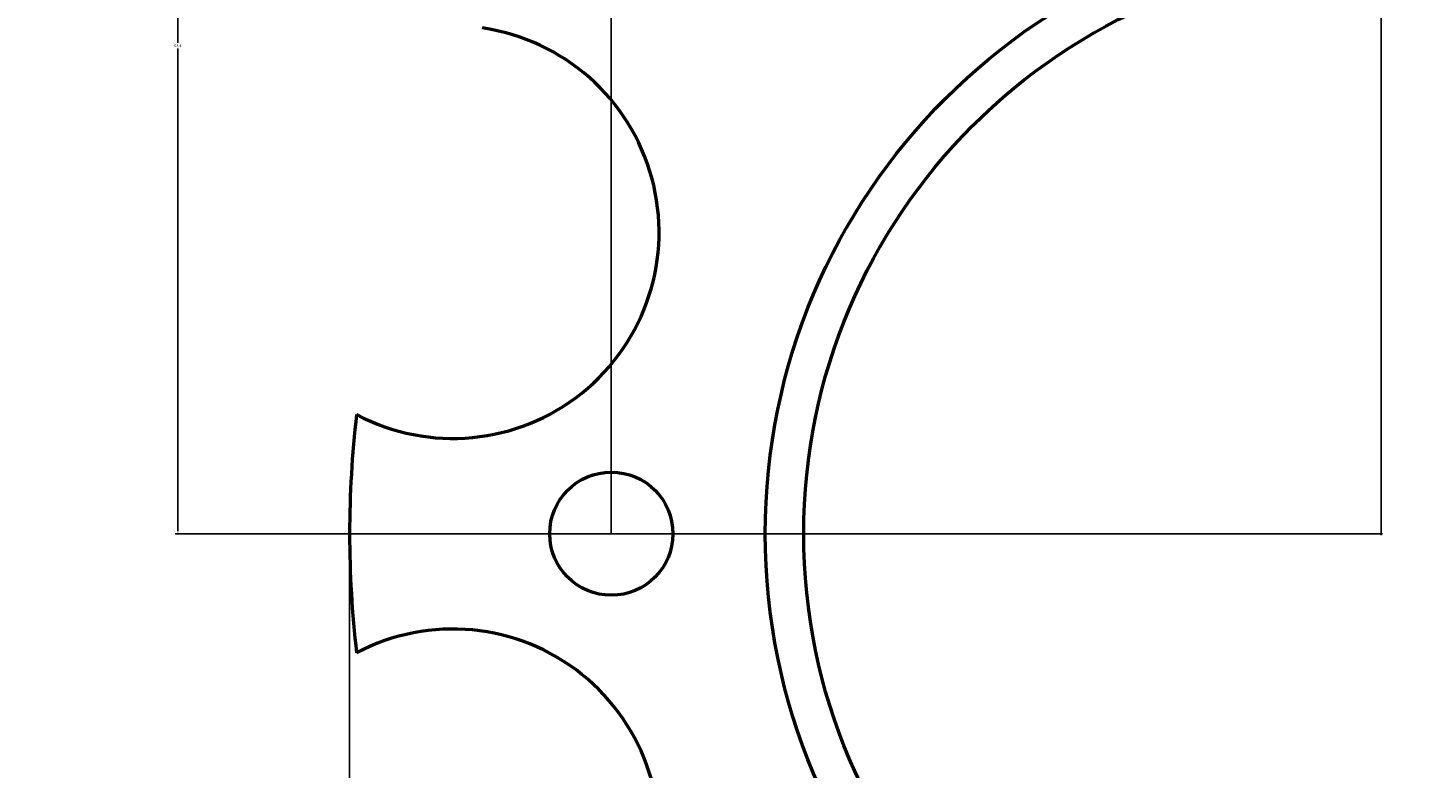
# Model space of a CAD drawing. Units: inches. Extents: x -62 to 104, y -63 to 91.
# Tile 2 of 4: x -62 to 29, y -1 to 47. Entities that reach past the tile are written whole.
import ezdxf

# ---------------------------------------------------------------- set-up
doc = ezdxf.new("R2010")
doc.units = ezdxf.units.IN
doc.header["$MEASUREMENT"] = 0
doc.layers.add('M-DIMS', color=2, linetype='Continuous', lineweight=18)
doc.layers.add('M-OUTL', color=7, linetype='Continuous', lineweight=50)
doc.styles.get("Standard").update_dxf_attribs({"font": 'arial.ttf'})
doc.dimstyles.get("Standard").update_dxf_attribs({"dimtxt": 0.18, "dimasz": 0.18, "dimexe": 0.18, "dimexo": 0.0625, "dimgap": 0.09, "dimtad": 0, "dimtih": 1, "dimtoh": 1, "dimdec": 4, "dimzin": 0, "dimdsep": 46, "dimtxsty": 'Standard', "dimcen": 0.09, "dimadec": 0, "dimazin": 0, "dimtfac": 1, "dimtdec": 4, "dimtofl": 0, "dimtmove": 0, "dimatfit": 3, "dimfxl": 1, "dimtolj": 1, "dimtzin": 0, "dimarcsym": 0})

# ---------------------------------------------------------------- blocks, each defined once
blk = doc.blocks.new('BOLT-HOLE-D8')
blk.add_circle((4, 4), 4)
blk = doc.blocks.new('*D2')
at = {"layer": 'Defpoints', "color": 0, "transparency": 16777216}
for p in [(-41.548, 13.739), (92.452, 13.739), (92.452, -63.102)]:
    blk.add_point(p, dxfattribs=at)
at = {"layer": 'M-DIMS', "color": 0, "lineweight": -2, "transparency": 16777216}
for p, q in [((-41.548, 13.677), (-41.548, -63.282)), ((92.452, 13.677), (92.452, -63.282)), ((-41.368, -63.102), (25.172, -63.102)), ((92.272, -63.102), (25.732, -63.102))]:
    blk.add_line(p, q, dxfattribs=at)
at = {"layer": 'M-DIMS', "color": 0, "transparency": 16777216}
for points in [[(-41.368, -63.072), (-41.368, -63.132), (-41.548, -63.102)], [(92.272, -63.072), (92.272, -63.132), (92.452, -63.102)]]:
    blk.add_solid(points, dxfattribs=at)
at = {"layer": 'M-DIMS', "color": 0, "transparency": 16777216, "insert": (25.452, -63.102), "char_height": 0.18, "attachment_point": 5}
blk.add_mtext('\\A1;134', dxfattribs=at)
blk = doc.blocks.new('*D4')
at = {"layer": 'Defpoints', "color": 0, "transparency": 16777216}
for p in [(25.452, 90.58), (-24.548, 13.739), (25.452, 13.739)]:
    blk.add_point(p, dxfattribs=at)
at = {"layer": 'M-DIMS', "color": 0, "lineweight": -2, "transparency": 16777216}
for p, q in [((-24.548, 13.802), (-24.548, 90.76)), ((-24.368, 90.58), (0.233, 90.58)), ((25.272, 90.58), (0.671, 90.58)), ((25.452, 13.802), (25.452, 90.76))]:
    blk.add_line(p, q, dxfattribs=at)
at = {"layer": 'M-DIMS', "color": 0, "transparency": 16777216}
for points in [[(-24.368, 90.61), (-24.368, 90.55), (-24.548, 90.58)], [(25.272, 90.61), (25.272, 90.55), (25.452, 90.58)]]:
    blk.add_solid(points, dxfattribs=at)
at = {"layer": 'M-DIMS', "color": 0, "transparency": 16777216, "insert": (0.452, 90.58), "char_height": 0.18, "attachment_point": 5}
blk.add_mtext('\\A1;50', dxfattribs=at)
blk = doc.blocks.new('*D5')
at = {"layer": 'Defpoints', "color": 0, "transparency": 16777216}
for p in [(-52.703, 77.139), (25.452, 77.139), (25.452, 13.739)]:
    blk.add_point(p, dxfattribs=at)
at = {"layer": 'M-DIMS', "color": 0, "lineweight": -2, "transparency": 16777216}
for p, q in [((25.389, 77.139), (-52.883, 77.139)), ((-52.703, 76.959), (-52.703, 45.621)), ((-52.703, 13.919), (-52.703, 45.257)), ((25.389, 13.739), (-52.883, 13.739))]:
    blk.add_line(p, q, dxfattribs=at)
at = {"layer": 'M-DIMS', "color": 0, "transparency": 16777216}
for points in [[(-52.733, 76.959), (-52.673, 76.959), (-52.703, 77.139)], [(-52.733, 13.919), (-52.673, 13.919), (-52.703, 13.739)]]:
    blk.add_solid(points, dxfattribs=at)
at = {"layer": 'M-DIMS', "color": 0, "transparency": 16777216, "insert": (-52.703, 45.439), "char_height": 0.18, "attachment_point": 5}
blk.add_mtext('\\A1;63.4', dxfattribs=at)
blk = doc.blocks.new('*D6')
at = {"layer": 'Defpoints', "color": 0, "transparency": 16777216}
for p in [(-28.752, 53.121), (25.452, 13.739)]:
    blk.add_point(p, dxfattribs=at)
at = {"layer": 'M-DIMS', "color": 0, "lineweight": -2, "transparency": 16777216}
for p, q in [((-61.454, 76.75), (-61.274, 76.75)), ((-61.274, 76.75), (-28.898, 53.227)), ((25.362, 13.739), (25.542, 13.739)), ((25.452, 13.649), (25.452, 13.829))]:
    blk.add_line(p, q, dxfattribs=at)
at = {"layer": 'M-DIMS', "color": 0, "transparency": 16777216}
blk.add_solid([(-28.88, 53.251), (-28.915, 53.203), (-28.752, 53.121)], dxfattribs=at)
at = {"layer": 'M-DIMS', "color": 0, "transparency": 16777216, "insert": (-62.014, 76.75), "char_height": 0.18, "attachment_point": 5}
blk.add_mtext('\\A1;10X R67', dxfattribs=at)
blk = doc.blocks.new('*D8')
at = {"layer": 'Defpoints', "color": 0, "transparency": 16777216}
for p in [(63.04, 27.42), (-12.136, 0.059)]:
    blk.add_point(p, dxfattribs=at)
at = {"layer": 'M-DIMS', "color": 0, "lineweight": -2, "transparency": 16777216}
for p, q in [((85.592, 35.628), (63.209, 27.481)), ((85.772, 35.628), (85.592, 35.628)), ((25.362, 13.739), (25.542, 13.739)), ((25.452, 13.649), (25.452, 13.829))]:
    blk.add_line(p, q, dxfattribs=at)
at = {"layer": 'M-DIMS', "color": 0, "transparency": 16777216}
blk.add_solid([(63.199, 27.51), (63.219, 27.453), (63.04, 27.42)], dxfattribs=at)
at = {"layer": 'M-DIMS', "color": 0, "transparency": 16777216, "insert": (86.089, 35.628), "char_height": 0.18, "attachment_point": 5}
blk.add_mtext('\\A1;∅80', dxfattribs=at)
blk = doc.blocks.new('*D9')
at = {"layer": 'Defpoints', "color": 0, "transparency": 16777216}
for p in [(57.928, 32.489), (-7.024, -5.011)]:
    blk.add_point(p, dxfattribs=at)
at = {"layer": 'M-DIMS', "color": 0, "lineweight": -2, "transparency": 16777216}
for p, q in [((25.362, 13.739), (25.542, 13.739)), ((25.452, 13.649), (25.452, 13.829)), ((-26.509, -16.261), (-7.18, -5.101)), ((-26.689, -16.261), (-26.509, -16.261))]:
    blk.add_line(p, q, dxfattribs=at)
at = {"layer": 'M-DIMS', "color": 0, "transparency": 16777216}
blk.add_solid([(-7.195, -5.075), (-7.165, -5.127), (-7.024, -5.011)], dxfattribs=at)
at = {"layer": 'M-DIMS', "color": 0, "transparency": 16777216, "insert": (-27.007, -16.261), "char_height": 0.18, "attachment_point": 5}
blk.add_mtext('\\A1;∅75', dxfattribs=at)

msp = doc.modelspace()

# ---------------------------------------------------------------- linework, layer by layer
at = {"layer": 'M-OUTL'}
for radius in [40, 37.5]:
    msp.add_circle((25.452, 13.739), radius, dxfattribs=at)
for centre, radius, start, end in [((-34.845, 33.331), 13.4, 242.17695, 81.82305), ((25.452, 13.739), 67, 173.36555, 186.63445), ((-34.845, -5.852), 13.4, 278.17695, 117.82305)]:
    msp.add_arc(centre, radius, start, end, dxfattribs=at)

# ---------------------------------------------------------------- block references
msp.add_blockref('BOLT-HOLE-D8', (-28.548, 9.739), dxfattribs=at)

# ---------------------------------------------------------------- dimensions: what is measured, and where the dimension line sits
at = {"layer": 'M-DIMS'}
for base, p1, p2, picture, middle in [((25.452, 90.58), (-24.548, 13.739), (25.452, 13.739), '*D4', (0.452, 90.58)), ((92.452, -63.102), (-41.548, 13.739), (92.452, 13.739), '*D2', (25.452, -63.102))]:
    dim = msp.add_linear_dim(base=base, p1=p1, p2=p2, dimstyle='Standard', override={"dimdec": 0, "dimlfac": 1, "dimrnd": 0, "dimzin": 0, "dimdsep": 46, "dimlunit": 2}, dxfattribs=at)
    dim.commit()
    dim.dimension.update_dxf_attribs({"geometry": picture, "text_midpoint": middle})
dim = msp.add_radius_dim(center=(25.452, 13.739), mpoint=(-28.752, 53.121), text='10X <>', dimstyle='Standard', override={"dimdec": 0, "dimlfac": 1, "dimrnd": 0, "dimzin": 0, "dimdsep": 46, "dimlunit": 2}, dxfattribs=at)
dim.commit()
dim.dimension.update_dxf_attribs({"geometry": '*D6', "text_midpoint": (-62.014, 76.75), "dimtype": 164})
dim = msp.add_linear_dim(base=(-52.703, 77.139), p1=(25.452, 13.739), p2=(25.452, 77.139), angle=90, dimstyle='Standard', override={"dimdec": 1, "dimlfac": 1, "dimrnd": 0, "dimzin": 0, "dimdsep": 46, "dimlunit": 2}, dxfattribs=at)
dim.commit()
dim.dimension.update_dxf_attribs({"geometry": '*D5', "text_midpoint": (-52.703, 45.439)})
for p1, p2, picture, middle in [((-12.136, 0.059), (63.04, 27.42), '*D8', (86.089, 35.628)), ((57.928, 32.489), (-7.024, -5.011), '*D9', (-27.007, -16.261))]:
    dim = msp.add_diameter_dim_2p(p1=p1, p2=p2, dimstyle='Standard', override={"dimdec": 0, "dimlfac": 1, "dimrnd": 0, "dimzin": 0, "dimdsep": 46, "dimlunit": 2}, dxfattribs=at)
    dim.commit()
    dim.dimension.update_dxf_attribs({"geometry": picture, "text_midpoint": middle, "dimtype": 163})

doc.saveas('drawing.dxf')
